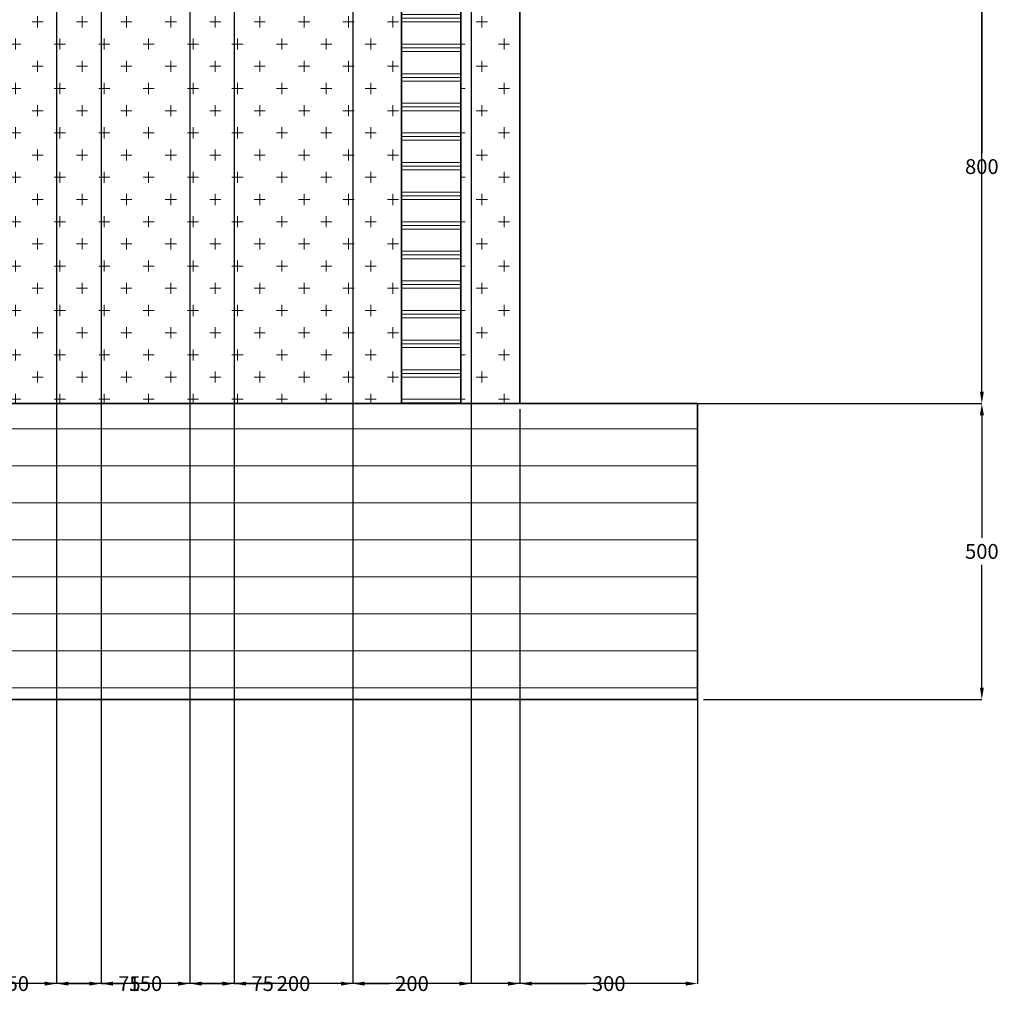
# Model space of a CAD drawing. Units: millimetres. Extents: x -692 to 9639, y -141 to 10345.
# Tile 7 of 19: x 7929 to 9592, y -141 to 1504. Entities that reach past the tile are written whole.
import ezdxf

# ---------------------------------------------------------------- set-up
doc = ezdxf.new("R2010")
doc.units = ezdxf.units.MM
doc.header["$MEASUREMENT"] = 0
for name, color, linetype, lineweight in [('A-ANNO-DIMS', 2, 'Continuous', 18), ('A-ELEV', 7, 'Continuous', 35), ('A-ELEV-PATT', 8, 'Continuous', 13)]:
    doc.layers.add(name, color=color, linetype=linetype, lineweight=lineweight)
doc.styles.get("Standard").update_dxf_attribs({"font": 'arial.ttf'})
doc.dimstyles.get("Standard").update_dxf_attribs({"dimtxt": 25, "dimasz": 20, "dimexe": 0.18, "dimexo": 10, "dimgap": 10, "dimtad": 0, "dimtih": 1, "dimtoh": 1, "dimdec": 0, "dimzin": 0, "dimdsep": 46, "dimtxsty": 'Standard', "dimcen": 10, "dimadec": 0, "dimazin": 0, "dimtfac": 1, "dimtdec": 0, "dimtofl": 0, "dimtmove": 0, "dimatfit": 3, "dimfxl": 1, "dimtolj": 1, "dimtzin": 0, "dimarcsym": 0})

# ---------------------------------------------------------------- blocks, each defined once
blk = doc.blocks.new('*D6')
at = {"layer": 'A-ANNO-DIMS', "color": 0, "lineweight": -2, "transparency": 16777216}
for p, q in [((2473.7, 345.6), (2473.7, -124.6)), ((9073.7, 345.6), (9073.7, -124.6)), ((2493.7, -124.4), (5726.4, -124.4)), ((9053.7, -124.4), (5821.1, -124.4))]:
    blk.add_line(p, q, dxfattribs=at)
at = {"layer": 'A-ANNO-DIMS', "color": 0, "lineweight": -3, "transparency": 16777216}
for points in [[(2493.7, -121.1), (2493.7, -127.8), (2473.7, -124.4)], [(9053.7, -121.1), (9053.7, -127.8), (9073.7, -124.4)]]:
    blk.add_solid(points, dxfattribs=at)
at = {"layer": 'Defpoints', "color": 0, "lineweight": -3, "transparency": 16777216}
for p in [(2473.7, 355.6), (9073.7, 355.6), (9073.7, -124.4)]:
    blk.add_point(p, dxfattribs=at)
at = {"layer": 'A-ANNO-DIMS', "color": 0, "transparency": 16777216, "insert": (5773.7, -124.4), "char_height": 25, "attachment_point": 5}
blk.add_mtext('\\A1;6600', dxfattribs=at)
blk = doc.blocks.new('*D7')
at = {"layer": 'A-ANNO-DIMS', "color": 0, "lineweight": -2, "transparency": 16777216}
for p, q in [((8481.5, 9848.8), (-649.1, 9848.8)), ((-648.9, 9828.8), (-648.9, 5124.9)), ((-648.9, 375.6), (-648.9, 5079.4)), ((2463.7, 355.6), (-649.1, 355.6))]:
    blk.add_line(p, q, dxfattribs=at)
at = {"layer": 'A-ANNO-DIMS', "color": 0, "lineweight": -3, "transparency": 16777216}
for points in [[(-652.2, 9828.8), (-645.6, 9828.8), (-648.9, 9848.8)], [(-652.2, 375.6), (-645.6, 375.6), (-648.9, 355.6)]]:
    blk.add_solid(points, dxfattribs=at)
at = {"layer": 'Defpoints', "color": 0, "lineweight": -3, "transparency": 16777216}
for p in [(-648.9, 9848.8), (8491.5, 9848.8), (2473.7, 355.6)]:
    blk.add_point(p, dxfattribs=at)
at = {"layer": 'A-ANNO-DIMS', "color": 0, "transparency": 16777216, "insert": (-648.9, 5102.2), "char_height": 25, "attachment_point": 5}
blk.add_mtext('\\A1;9493', dxfattribs=at)
blk = doc.blocks.new('*D8')
at = {"layer": 'A-ANNO-DIMS', "color": 0, "lineweight": -2, "transparency": 16777216}
for p, q in [((9083.7, 855.6), (9553.9, 855.6)), ((9553.7, 835.6), (9553.7, 628.3)), ((9553.7, 375.6), (9553.7, 582.8)), ((9083.7, 355.6), (9553.9, 355.6))]:
    blk.add_line(p, q, dxfattribs=at)
at = {"layer": 'A-ANNO-DIMS', "color": 0, "lineweight": -3, "transparency": 16777216}
for points in [[(9550.4, 835.6), (9557.1, 835.6), (9553.7, 855.6)], [(9550.4, 375.6), (9557.1, 375.6), (9553.7, 355.6)]]:
    blk.add_solid(points, dxfattribs=at)
at = {"layer": 'Defpoints', "color": 0, "lineweight": -3, "transparency": 16777216}
for p in [(9073.7, 855.6), (9553.7, 855.6), (9073.7, 355.6)]:
    blk.add_point(p, dxfattribs=at)
at = {"layer": 'A-ANNO-DIMS', "color": 0, "transparency": 16777216, "insert": (9553.7, 605.6), "char_height": 25, "attachment_point": 5}
blk.add_mtext('\\A1;500', dxfattribs=at)
blk = doc.blocks.new('*D9')
at = {"layer": 'A-ANNO-DIMS', "color": 0, "lineweight": -2, "transparency": 16777216}
for p, q in [((8501.5, 8848.8), (9553.9, 8848.8)), ((9553.7, 8828.8), (9553.7, 4874.9)), ((9553.7, 875.6), (9553.7, 4829.4)), ((9083.7, 855.6), (9553.9, 855.6))]:
    blk.add_line(p, q, dxfattribs=at)
at = {"layer": 'A-ANNO-DIMS', "color": 0, "lineweight": -3, "transparency": 16777216}
for points in [[(9550.4, 8828.8), (9557.1, 8828.8), (9553.7, 8848.8)], [(9550.4, 875.6), (9557.1, 875.6), (9553.7, 855.6)]]:
    blk.add_solid(points, dxfattribs=at)
at = {"layer": 'Defpoints', "color": 0, "lineweight": -3, "transparency": 16777216}
for p in [(8491.5, 8848.8), (9553.7, 8848.8), (9073.7, 855.6)]:
    blk.add_point(p, dxfattribs=at)
at = {"layer": 'A-ANNO-DIMS', "color": 0, "transparency": 16777216, "insert": (9553.7, 4852.2), "char_height": 25, "attachment_point": 5}
blk.add_mtext('\\A1;7993', dxfattribs=at)
blk = doc.blocks.new('*D23')
at = {"layer": 'A-ANNO-DIMS', "color": 0, "lineweight": -2, "transparency": 16777216}
for p, q in [((6891.7, 845.6), (6891.7, -124.6)), ((8773.7, 845.6), (8773.7, -124.6)), ((6911.7, -124.4), (7786.7, -124.4)), ((8753.7, -124.4), (7878.8, -124.4))]:
    blk.add_line(p, q, dxfattribs=at)
at = {"layer": 'A-ANNO-DIMS', "color": 0, "lineweight": -3, "transparency": 16777216}
for points in [[(6911.7, -121.1), (6911.7, -127.8), (6891.7, -124.4)], [(8753.7, -121.1), (8753.7, -127.8), (8773.7, -124.4)]]:
    blk.add_solid(points, dxfattribs=at)
at = {"layer": 'Defpoints', "color": 0, "lineweight": -3, "transparency": 16777216}
for p in [(6891.7, 855.6), (8773.7, 855.6), (8773.7, -124.4)]:
    blk.add_point(p, dxfattribs=at)
at = {"layer": 'A-ANNO-DIMS', "color": 0, "transparency": 16777216, "insert": (7832.7, -124.4), "char_height": 25, "attachment_point": 5}
blk.add_mtext('\\A1;1882', dxfattribs=at)
blk = doc.blocks.new('*D24')
at = {"layer": 'A-ANNO-DIMS', "color": 0, "lineweight": -2, "transparency": 16777216}
for p, q in [((8773.7, 845.6), (8773.7, -124.6)), ((9073.7, 845.6), (9073.7, -124.6)), ((8793.7, -124.4), (8886.2, -124.4)), ((9053.7, -124.4), (8961.3, -124.4))]:
    blk.add_line(p, q, dxfattribs=at)
at = {"layer": 'A-ANNO-DIMS', "color": 0, "lineweight": -3, "transparency": 16777216}
for points in [[(8793.7, -121.1), (8793.7, -127.8), (8773.7, -124.4)], [(9053.7, -121.1), (9053.7, -127.8), (9073.7, -124.4)]]:
    blk.add_solid(points, dxfattribs=at)
at = {"layer": 'Defpoints', "color": 0, "lineweight": -3, "transparency": 16777216}
for p in [(8773.7, 855.6), (9073.7, 855.6), (9073.7, -124.4)]:
    blk.add_point(p, dxfattribs=at)
at = {"layer": 'A-ANNO-DIMS', "color": 0, "transparency": 16777216, "insert": (8923.7, -124.4), "char_height": 25, "attachment_point": 5}
blk.add_mtext('\\A1;300', dxfattribs=at)
blk = doc.blocks.new('*D28')
at = {"layer": 'A-ANNO-DIMS', "color": 0, "lineweight": -2, "transparency": 16777216}
for p, q in [((8583.7, 1655.6), (9553.9, 1655.6)), ((9553.7, 1635.6), (9553.7, 1278.3)), ((9553.7, 875.6), (9553.7, 1232.8)), ((8583.7, 855.6), (9553.9, 855.6))]:
    blk.add_line(p, q, dxfattribs=at)
at = {"layer": 'A-ANNO-DIMS', "color": 0, "lineweight": -3, "transparency": 16777216}
for points in [[(9550.4, 1635.6), (9557.1, 1635.6), (9553.7, 1655.6)], [(9550.4, 875.6), (9557.1, 875.6), (9553.7, 855.6)]]:
    blk.add_solid(points, dxfattribs=at)
at = {"layer": 'Defpoints', "color": 0, "lineweight": -3, "transparency": 16777216}
for p in [(8573.7, 1655.6), (9553.7, 1655.6), (8573.7, 855.6)]:
    blk.add_point(p, dxfattribs=at)
at = {"layer": 'A-ANNO-DIMS', "color": 0, "transparency": 16777216, "insert": (9553.7, 1255.6), "char_height": 25, "attachment_point": 5}
blk.add_mtext('\\A1;800', dxfattribs=at)
blk = doc.blocks.new('*D46')
at = {"layer": 'A-ANNO-DIMS', "color": 0, "lineweight": -2, "transparency": 16777216}
for p, q in [((7841.5, 3138.3), (7841.5, -124.6)), ((7991.5, 3138.3), (7991.5, -124.6)), ((7861.5, -124.4), (7880.1, -124.4)), ((7971.5, -124.4), (7952.9, -124.4))]:
    blk.add_line(p, q, dxfattribs=at)
at = {"layer": 'A-ANNO-DIMS', "color": 0, "lineweight": -3, "transparency": 16777216}
for points in [[(7861.5, -121.1), (7861.5, -127.8), (7841.5, -124.4)], [(7971.5, -121.1), (7971.5, -127.8), (7991.5, -124.4)]]:
    blk.add_solid(points, dxfattribs=at)
at = {"layer": 'Defpoints', "color": 0, "lineweight": -3, "transparency": 16777216}
for p in [(7841.5, 3148.3), (7991.5, 3148.3), (7991.5, -124.4)]:
    blk.add_point(p, dxfattribs=at)
at = {"layer": 'A-ANNO-DIMS', "color": 0, "transparency": 16777216, "insert": (7916.5, -124.4), "char_height": 25, "attachment_point": 5}
blk.add_mtext('\\A1;150', dxfattribs=at)
blk = doc.blocks.new('*D47')
at = {"layer": 'A-ANNO-DIMS', "color": 0, "lineweight": -2, "transparency": 16777216}
for p, q in [((7991.5, 3138.3), (7991.5, -124.6)), ((8066.5, 3138.3), (8066.5, -124.6)), ((8011.5, -124.4), (8046.5, -124.4)), ((8066.5, -124.4), (8086.5, -124.4))]:
    blk.add_line(p, q, dxfattribs=at)
at = {"layer": 'A-ANNO-DIMS', "color": 0, "lineweight": -3, "transparency": 16777216}
for points in [[(8011.5, -121.1), (8011.5, -127.8), (7991.5, -124.4)], [(8046.5, -121.1), (8046.5, -127.8), (8066.5, -124.4)]]:
    blk.add_solid(points, dxfattribs=at)
at = {"layer": 'Defpoints', "color": 0, "lineweight": -3, "transparency": 16777216}
for p in [(7991.5, 3148.3), (8066.5, 3148.3), (8066.5, -124.4)]:
    blk.add_point(p, dxfattribs=at)
at = {"layer": 'A-ANNO-DIMS', "color": 0, "transparency": 16777216, "insert": (8114.4, -124.4), "char_height": 25, "attachment_point": 5}
blk.add_mtext('\\A1;75', dxfattribs=at)
blk = doc.blocks.new('*D48')
at = {"layer": 'A-ANNO-DIMS', "color": 0, "lineweight": -2, "transparency": 16777216}
for p, q in [((8066.5, 3138.3), (8066.5, -124.6)), ((8216.5, 3138.3), (8216.5, -124.6)), ((8086.5, -124.4), (8105.1, -124.4)), ((8196.5, -124.4), (8177.9, -124.4))]:
    blk.add_line(p, q, dxfattribs=at)
at = {"layer": 'A-ANNO-DIMS', "color": 0, "lineweight": -3, "transparency": 16777216}
for points in [[(8086.5, -121.1), (8086.5, -127.8), (8066.5, -124.4)], [(8196.5, -121.1), (8196.5, -127.8), (8216.5, -124.4)]]:
    blk.add_solid(points, dxfattribs=at)
at = {"layer": 'Defpoints', "color": 0, "lineweight": -3, "transparency": 16777216}
for p in [(8066.5, 3148.3), (8216.5, 3148.3), (8216.5, -124.4)]:
    blk.add_point(p, dxfattribs=at)
at = {"layer": 'A-ANNO-DIMS', "color": 0, "transparency": 16777216, "insert": (8141.5, -124.4), "char_height": 25, "attachment_point": 5}
blk.add_mtext('\\A1;150', dxfattribs=at)
blk = doc.blocks.new('*D49')
at = {"layer": 'A-ANNO-DIMS', "color": 0, "lineweight": -2, "transparency": 16777216}
for p, q in [((8216.5, 3138.3), (8216.5, -124.6)), ((8291.5, 3138.3), (8291.5, -124.6)), ((8236.5, -124.4), (8271.5, -124.4)), ((8291.5, -124.4), (8311.5, -124.4))]:
    blk.add_line(p, q, dxfattribs=at)
at = {"layer": 'A-ANNO-DIMS', "color": 0, "lineweight": -3, "transparency": 16777216}
for points in [[(8236.5, -121.1), (8236.5, -127.8), (8216.5, -124.4)], [(8271.5, -121.1), (8271.5, -127.8), (8291.5, -124.4)]]:
    blk.add_solid(points, dxfattribs=at)
at = {"layer": 'Defpoints', "color": 0, "lineweight": -3, "transparency": 16777216}
for p in [(8216.5, 3148.3), (8291.5, 3148.3), (8291.5, -124.4)]:
    blk.add_point(p, dxfattribs=at)
at = {"layer": 'A-ANNO-DIMS', "color": 0, "transparency": 16777216, "insert": (8339.4, -124.4), "char_height": 25, "attachment_point": 5}
blk.add_mtext('\\A1;75', dxfattribs=at)
blk = doc.blocks.new('*D50')
at = {"layer": 'A-ANNO-DIMS', "color": 0, "lineweight": -2, "transparency": 16777216}
for p, q in [((8291.5, 3138.3), (8291.5, -124.6)), ((8491.5, 3138.3), (8491.5, -124.6)), ((8311.5, -124.4), (8353.8, -124.4)), ((8471.5, -124.4), (8429.3, -124.4))]:
    blk.add_line(p, q, dxfattribs=at)
at = {"layer": 'A-ANNO-DIMS', "color": 0, "lineweight": -3, "transparency": 16777216}
for points in [[(8311.5, -121.1), (8311.5, -127.8), (8291.5, -124.4)], [(8471.5, -121.1), (8471.5, -127.8), (8491.5, -124.4)]]:
    blk.add_solid(points, dxfattribs=at)
at = {"layer": 'Defpoints', "color": 0, "lineweight": -3, "transparency": 16777216}
for p in [(8291.5, 3148.3), (8491.5, 3148.3), (8491.5, -124.4)]:
    blk.add_point(p, dxfattribs=at)
at = {"layer": 'A-ANNO-DIMS', "color": 0, "transparency": 16777216, "insert": (8391.5, -124.4), "char_height": 25, "attachment_point": 5}
blk.add_mtext('\\A1;200', dxfattribs=at)
blk = doc.blocks.new('*D51')
at = {"layer": 'A-ANNO-DIMS', "color": 0, "lineweight": -2, "transparency": 16777216}
for p, q in [((8691.5, 4838.8), (8691.5, -124.6)), ((8491.5, 3138.3), (8491.5, -124.6)), ((8511.5, -124.4), (8553.8, -124.4)), ((8671.5, -124.4), (8629.3, -124.4))]:
    blk.add_line(p, q, dxfattribs=at)
at = {"layer": 'A-ANNO-DIMS', "color": 0, "lineweight": -3, "transparency": 16777216}
for points in [[(8511.5, -121.1), (8511.5, -127.8), (8491.5, -124.4)], [(8671.5, -121.1), (8671.5, -127.8), (8691.5, -124.4)]]:
    blk.add_solid(points, dxfattribs=at)
at = {"layer": 'Defpoints', "color": 0, "lineweight": -3, "transparency": 16777216}
for p in [(8691.5, 4848.8), (8491.5, 3148.3), (8691.5, -124.4)]:
    blk.add_point(p, dxfattribs=at)
at = {"layer": 'A-ANNO-DIMS', "color": 0, "transparency": 16777216, "insert": (8591.5, -124.4), "char_height": 25, "attachment_point": 5}
blk.add_mtext('\\A1;200', dxfattribs=at)

msp = doc.modelspace()

# ---------------------------------------------------------------- hatches: boundary and pattern name
at = {"layer": 'A-ELEV-PATT'}
h = msp.add_hatch(dxfattribs=at)
h.set_pattern_fill('CROSS', color=256, scale=150)
h.paths.add_polyline_path([(8573.746, 1655.575), (7091.746, 1655.575), (7091.746, 855.575), (7273.746, 855.575), (8573.746, 855.575)], flags=17)
h.paths.add_polyline_path([(8773.746, 1855.575), (8463.966, 1855.575), (8463.828, 1855.268), (8463.709, 1855.575), (7761.103, 1855.575), (7760.965, 1855.268), (7760.846, 1855.575), (7409.705, 1855.575), (7409.567, 1855.268), (7409.448, 1855.575), (7076.174, 1855.575), (7076.035, 1855.268), (7075.916, 1855.575), (6891.746, 1855.575), (6891.746, 855.575), (6991.746, 855.575), (6991.746, 1755.575), (8673.746, 1755.575), (8673.746, 855.575), (8773.746, 855.575)])
h = msp.add_hatch(dxfattribs=at)
h.set_pattern_fill('PLAST', color=256, scale=200)
h.paths.add_polyline_path([(8673.746, 1755.575), (6991.746, 1755.575), (6991.746, 855.575), (7091.746, 855.575), (7091.746, 1655.575), (8573.746, 1655.575), (8573.746, 855.575), (8673.746, 855.575)])
h = msp.add_hatch(dxfattribs=at)
h.set_pattern_fill('LINE', color=256, scale=500)
h.paths.add_polyline_path([(9073.746, 855.575), (8773.746, 855.575), (7273.746, 855.575), (2773.746, 855.575), (2473.746, 855.575), (2473.746, 355.575), (9073.746, 355.575)])

# ---------------------------------------------------------------- linework, layer by layer
at = {"layer": 'A-ELEV'}
for p, q in [((8773.746, 1855.575), (8773.746, 855.575)), ((8673.746, 1755.575), (8673.746, 855.575)), ((8573.746, 1655.575), (8573.746, 855.575)), ((7273.746, 855.575), (8773.746, 855.575)), ((9073.746, 855.575), (8773.746, 855.575)), ((9073.746, 355.575), (9073.746, 855.575)), ((2473.746, 355.575), (9073.746, 355.575))]:
    msp.add_line(p, q, dxfattribs=at)

# ---------------------------------------------------------------- dimensions: what is measured, and where the dimension line sits
at = {"layer": 'A-ANNO-DIMS'}
for base, p1, p2, picture, middle in [((-648.912, 9848.772), (2473.746, 355.575), (8491.547, 9848.772), '*D7', (-648.912, 5102.173)), ((9553.746, 8848.772), (9073.746, 855.575), (8491.547, 8848.772), '*D9', (9553.746, 4852.173)), ((9553.746, 1655.575), (8573.746, 855.575), (8573.746, 1655.575), '*D28', (9553.746, 1255.575)), ((9553.746, 855.575), (9073.746, 355.575), (9073.746, 855.575), '*D8', (9553.746, 605.575))]:
    dim = msp.add_linear_dim(base=base, p1=p1, p2=p2, angle=90, dimstyle='Standard', override={"dimdec": 0, "dimlfac": 1, "dimrnd": 0, "dimzin": 0, "dimdsep": 46, "dimlunit": 2}, dxfattribs=at)
    dim.commit()
    dim.dimension.update_dxf_attribs({"geometry": picture, "text_midpoint": middle})
for base, p1, p2, picture, middle in [((8691.547, -124.425), (8491.547, 3148.27), (8691.547, 4848.772), '*D51', (8591.547, -124.425)), ((7991.547, -124.425), (7841.547, 3148.27), (7991.547, 3148.27), '*D46', (7916.547, -124.425)), ((8066.547, -124.425), (7991.547, 3148.27), (8066.547, 3148.27), '*D47', (8114.444, -124.425)), ((8216.547, -124.425), (8066.547, 3148.27), (8216.547, 3148.27), '*D48', (8141.547, -124.425)), ((8291.547, -124.425), (8216.547, 3148.27), (8291.547, 3148.27), '*D49', (8339.444, -124.425)), ((8491.547, -124.425), (8291.547, 3148.27), (8491.547, 3148.27), '*D50', (8391.547, -124.425)), ((8773.746, -124.425), (6891.746, 855.575), (8773.746, 855.575), '*D23', (7832.746, -124.425)), ((9073.746, -124.425), (8773.746, 855.575), (9073.746, 855.575), '*D24', (8923.746, -124.425)), ((9073.746, -124.425), (2473.746, 355.575), (9073.746, 355.575), '*D6', (5773.746, -124.425))]:
    dim = msp.add_linear_dim(base=base, p1=p1, p2=p2, dimstyle='Standard', override={"dimdec": 0, "dimlfac": 1, "dimrnd": 0, "dimzin": 0, "dimdsep": 46, "dimlunit": 2}, dxfattribs=at)
    dim.commit()
    dim.dimension.update_dxf_attribs({"geometry": picture, "text_midpoint": middle})

doc.saveas('drawing.dxf')
